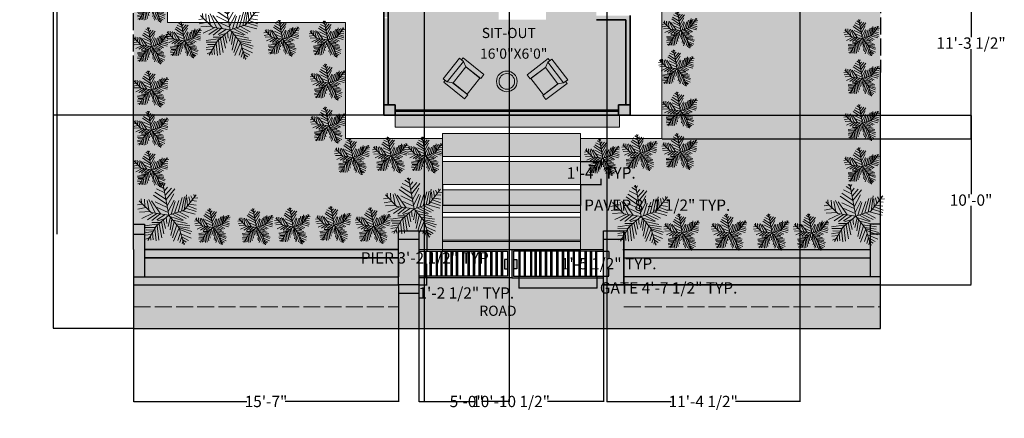
# Model space of a CAD drawing. Units: inches. Extents: x 853 to 1550, y 485 to 1596.
# Tile 1 of 18: x 853 to 1550, y 485 to 768. Entities that reach past the tile are written whole.
import ezdxf

# ---------------------------------------------------------------- set-up
doc = ezdxf.new("R2010")
doc.units = ezdxf.units.IN
doc.header["$MEASUREMENT"] = 0
doc.linetypes.add('ACAD_ISO02W100', pattern=[15, 12, -3])
for name, color, linetype, lineweight in [('A-ANNO-DIMS', 2, 'Continuous', 18), ('A-ANNO-TEXT', 250, 'Continuous', 25), ('A-AREA-IDEN', 250, 'Continuous', 18), ('A-WALL-PATT', 250, 'Continuous', 13), ('C-PROP', 8, 'ACAD_ISO02W100', 25), ('C-ROAD', 8, 'Continuous', 25), ('C-ROAD-MRKG', 7, 'ACAD_ISO02W100', 18), ('furniture', 250, 'Continuous', 18), ('L-GATE-PATT', 250, 'Continuous', 13), ('L-PAVE', 8, 'Continuous', 18), ('L-PLNT-TREE', 106, 'Continuous', 13), ('L-SITE-GATE', 250, 'Continuous', 25), ('L-SITE-WALL', 8, 'Continuous', 30), ('lawn', 106, 'Continuous', 18), ('walls', 250, 'Continuous', 35)]:
    doc.layers.add(name, color=color, linetype=linetype, lineweight=lineweight)
for name, color, linetype, lineweight, true_color in [('A-FLOR-PATT', 254, 'Continuous', 13, 0xfeeab9), ('A-FURN-PATT', 254, 'Continuous', 13, 0xfeeab9), ('C-ROAD-PATT', 250, 'Continuous', 13, 0x3d3d3d), ('L-PAVE-PATT', 9, 'Continuous', 13, 0xc7c8ca), ('L-PLNT-PATT', 85, 'Continuous', 13, 0x58ba48), ('L-SITE-WALL-PATT', 252, 'Continuous', 13, 0x939598)]:
    doc.layers.add(name, color=color, linetype=linetype, lineweight=lineweight, true_color=true_color)
doc.styles.get("Standard").update_dxf_attribs({"font": 'arial.ttf'})
doc.dimstyles.get("Standard").update_dxf_attribs({"dimtxt": 8, "dimasz": 0.18, "dimexe": 0.18, "dimexo": 0.0625, "dimgap": 0.09, "dimtad": 0, "dimtih": 1, "dimtoh": 1, "dimzin": 0, "dimdsep": 46, "dimlunit": 3, "dimtxsty": 'Standard', "dimcen": 0.09, "dimadec": 0, "dimazin": 0, "dimtfac": 1, "dimtofl": 0, "dimtmove": 0, "dimatfit": 3, "dimfxl": 1, "dimtolj": 1, "dimtzin": 0, "dimarcsym": 0})

# ---------------------------------------------------------------- blocks, each defined once
blk = doc.blocks.new('FABRIC SOFA 1S')
at = {"layer": 'furniture'}
for p, q in [((0, -15.1), (0, 15.1)), ((6, 15.1), (0, 15.1)), ((3, 18.1), (34, 18.1)), ((3, 15.1), (3, 18.1)), ((6, -15.1), (6, 15.1)), ((12, 11.8), (6, 15.1)), ((11.3, 12.1), (34, 12.1)), ((34, 12.1), (34, 18.1)), ((6, -15.1), (0, -15.1)), ((3, -18.1), (3, -15.1)), ((3, -18.1), (34, -18.1)), ((6, -15.1), (12, -11.8)), ((11.3, -12.1), (34, -12.1)), ((34, -12.1), (34, -18.1))]:
    blk.add_line(p, q, dxfattribs=at)
blk.add_lwpolyline([(12, -11.8), (12, 11.8), (33, 11.8), (33, -11.8)], close=True, dxfattribs=at)
blk = doc.blocks.new('*U18')
for p, q in [((-8.737, 47.138), (-17.069, 52.711)), ((-10.186, 53.64), (-13.084, 55.962)), ((0, 0), (-10.5, 57)), ((-9.099, 51.782), (-6.563, 55.962)), ((-3.665, 19.273), (-27.574, 35.527)), ((-5.114, 28.097), (-24.676, 40.636)), ((-7.288, 39.707), (-21.778, 46.673)), ((-7.65, 43.423), (-2.578, 49.46)), ((-5.839, 35.992), (4.667, 48.067)), ((-5.114, 27.632), (10.463, 46.673)), ((-2.941, 16.486), (8.652, 37.85)), ((27, 9), (48, 36)), ((27.127, 9.056), (31.112, 35.992)), ((44.153, 36.456), (45.239, 32.741)), ((-47.498, 19.737), (-55.83, 18.344)), ((-31.5, 4.5), (-52.5, 25.5)), ((-48.585, 21.131), (-49.309, 29.026)), ((-43.513, 28.561), (-42.427, 15.558)), ((-38.442, 26.239), (-34.819, 7.663)), ((-35.544, 28.097), (-24.314, 3.947)), ((-14.533, 2.09), (-30.834, 25.31)), ((-24.314, 23.917), (-2.941, 13.7)), ((-1.129, 6.734), (9.014, 26.704)), ((3.942, 1.625), (11.187, 24.381)), ((10.101, 3.483), (17.708, 26.239)), ((16.259, 5.805), (23.142, 31.348)), ((22.055, 7.198), (27.489, 32.277)), ((31.836, 30.883), (32.561, 16.486)), ((35.096, 32.741), (37.27, 22.524)), ((36.183, 19.737), (48.137, 17.88)), ((38.719, 34.134), (41.979, 28.561)), ((40.53, 25.775), (48.862, 24.846)), ((43.791, 29.954), (51.036, 30.883)), ((-40.615, 13.7), (-55.105, 10.913)), ((-33.37, 6.269), (-52.207, 5.34)), ((-28.299, 3.483), (-47.86, -5.805)), ((-21.416, 3.018), (-38.079, -8.128)), ((0, 0), (-31.5, 4.5)), ((-15.982, 2.09), (-30.11, -9.521)), ((0, 0), (-22.5, -19.5)), ((-6.563, 1.161), (-21.416, -8.128)), ((-20.691, 13.7), (-1.129, 4.876)), ((0, 0), (27, 9)), ((0, 0), (18, -22.5)), ((6.478, 1.625), (26.04, -8.592)), ((11.187, 3.483), (30.749, -5.805)), ((18.07, 5.805), (35.096, -3.483)), ((24.229, 7.663), (46.688, 1.625)), ((29.662, 12.307), (48.137, 6.269)), ((33.285, 16.486), (48.862, 10.913)), ((-17.431, -15.094), (-42.789, -18.809)), ((-15.257, -12.772), (-30.11, -12.772)), ((-6.563, -5.805), (-19.967, -9.985)), ((-17.069, -15.094), (-12.721, -40.172)), ((-13.446, -11.378), (-8.737, -32.741)), ((-9.461, -8.592), (-6.201, -23.453)), ((-4.752, -3.483), (-3.665, -14.629)), ((2.493, -3.019), (-1.491, -20.202)), ((1.769, -2.555), (24.229, -9.521)), ((5.029, -6.27), (2.131, -25.775)), ((9.014, -11.378), (3.58, -35.992)), ((14.085, -16.951), (6.478, -40.172)), ((7.565, -9.056), (32.198, -14.629)), ((12.274, -15.094), (36.907, -18.809)), ((-28.299, -29.026), (-42.789, -31.348)), ((-24.314, -21.596), (-42.427, -22.06)), ((-30.834, -34.135), (-42.427, -35.528)), ((-26.849, -26.24), (-40.253, -25.775)), ((-22.5, -19.5), (-37.5, -45)), ((-29.023, -30.884), (-27.936, -43.887)), ((-25.038, -23.918), (-22.865, -45.281)), ((-20.691, -18.345), (-17.793, -44.352)), ((18.07, -22.524), (8.289, -45.745)), ((20.244, -30.419), (15.897, -44.816)), ((16.259, -19.738), (36.183, -22.989)), ((18, -22.5), (27, -52.5)), ((18.433, -22.524), (40.53, -29.026)), ((19.157, -25.311), (38.719, -33.206)), ((21.331, -32.741), (39.081, -40.636)), ((-34.457, -39.708), (-40.978, -42.494)), ((-32.646, -36.921), (-31.921, -44.352)), ((22.78, -37.85), (19.519, -48.532)), ((22.78, -38.314), (34.372, -44.816)), ((24.591, -45.745), (23.142, -50.854)), ((24.591, -43.423), (30.749, -47.603)), ((26.764, -49.925), (28.213, -50.854))]:
    blk.add_line(p, q)
blk = doc.blocks.new('*D23')
at = {"layer": 'A-ANNO-DIMS', "color": 0, "lineweight": -2, "transparency": 16777216}
for p, q in [((879.97, 1474.13), (879.75, 1474.13)), ((879.93, 1473.95), (879.93, 1049.11)), ((879.93, 615.92), (879.93, 1040.76)), ((879.97, 615.74), (879.75, 615.74))]:
    blk.add_line(p, q, dxfattribs=at)
at = {"layer": 'A-ANNO-DIMS', "color": 0, "transparency": 16777216}
for points in [[(879.9, 1473.95), (879.96, 1473.95), (879.93, 1474.13)], [(879.9, 615.92), (879.96, 615.92), (879.93, 615.74)]]:
    blk.add_solid(points, dxfattribs=at)
at = {"layer": 'Defpoints', "color": 0, "transparency": 16777216}
for p in [(880.03, 1474.13), (879.93, 615.74), (880.03, 615.74)]:
    blk.add_point(p, dxfattribs=at)
at = {"layer": 'A-ANNO-DIMS', "color": 0, "transparency": 16777216, "insert": (879.93, 1044.94), "char_height": 8, "attachment_point": 5}
blk.add_mtext("\\A1;60'", dxfattribs=at)
blk = doc.blocks.new('GATE-PICKET-PANEL')
for p, q in [((0, 17.73), (0, 0)), ((1.11, 0), (1.11, 17.73)), ((3.76, 17.73), (3.76, 0)), ((4.87, 0), (4.87, 17.73)), ((8.23, 17.73), (8.23, 0)), ((9.34, 0), (9.34, 17.73)), ((11.49, 17.73), (11.49, 0)), ((12.61, 0), (12.61, 17.73)), ((14.66, 17.73), (14.66, 0)), ((15.77, 0), (15.77, 17.73)), ((18.68, 17.73), (18.68, 0)), ((19.79, 0), (19.79, 17.73)), ((22.43, 17.73), (22.43, 0)), ((23.54, 0), (23.54, 17.73)), ((26.82, 17.73), (26.82, 0)), ((27.93, 0), (27.93, 17.73)), ((30.74, 17.73), (30.74, 0)), ((31.85, 0), (31.85, 17.73)), ((34.53, 17.73), (34.53, 0)), ((35.64, 0), (35.64, 17.73)), ((38.4, 17.73), (38.4, 0)), ((39.51, 0), (39.51, 17.73)), ((42.59, 17.73), (42.59, 0)), ((43.7, 0), (43.7, 17.73)), ((46.7, 17.73), (46.7, 0)), ((47.82, 0), (47.82, 17.73)), ((50.49, 17.73), (50.49, 0)), ((51.61, 0), (51.61, 17.73)), ((54.2, 17.73), (54.2, 0)), ((55.32, 0), (55.32, 17.73))]:
    blk.add_line(p, q)
blk = doc.blocks.new('GATE-PIER')
for p, q in [((0, 38.25), (14.43, 38.25)), ((0, 0), (0, 38.25)), ((14.43, 38.25), (14.43, 0)), ((0, 32.5), (14.43, 32.5)), ((14.43, 0), (0, 0))]:
    blk.add_line(p, q)
blk = doc.blocks.new('ENTRY-PAVER')
for p, q in [((0, 16.22), (97.66, 16.22)), ((0, 0), (0, 16.22)), ((0, 16.22), (97.66, 16.22)), ((0, 0), (0, 16.22)), ((97.66, 16.22), (97.66, 0)), ((97.66, 16.22), (97.66, 0)), ((97.66, 0), (0, 0)), ((97.66, 0), (0, 0))]:
    blk.add_line(p, q)
blk = doc.blocks.new('*D47')
at = {"layer": 'A-ANNO-DIMS', "color": 0, "lineweight": -2, "transparency": 16777216}
for p, q in [((1152.25, 650.83), (1152.25, 636.06)), ((1249.91, 650.83), (1249.91, 636.06)), ((1152.43, 636.24), (1249.73, 636.24)), ((1249.91, 636.24), (1250.09, 636.24))]:
    blk.add_line(p, q, dxfattribs=at)
at = {"layer": 'A-ANNO-DIMS', "color": 0, "transparency": 16777216}
for points in [[(1152.43, 636.27), (1152.43, 636.21), (1152.25, 636.24)], [(1249.73, 636.27), (1249.73, 636.21), (1249.91, 636.24)]]:
    blk.add_solid(points, dxfattribs=at)
at = {"layer": 'Defpoints', "color": 0, "transparency": 16777216}
for p in [(1152.25, 650.89), (1249.91, 650.89), (1249.91, 636.24)]:
    blk.add_point(p, dxfattribs=at)
at = {"layer": 'A-ANNO-DIMS', "color": 0, "transparency": 16777216, "insert": (1304.18, 636.24), "char_height": 8, "attachment_point": 5}
blk.add_mtext('\\A1;PAVER 8\'-1 1/2" TYP.', dxfattribs=at)
blk = doc.blocks.new('*D48')
at = {"layer": 'A-ANNO-DIMS', "color": 0, "lineweight": -2, "transparency": 16777216}
for p, q in [((1249.97, 667.11), (1264.74, 667.11)), ((1264.56, 666.93), (1264.56, 663.11)), ((1264.56, 651.07), (1264.56, 654.89)), ((1249.97, 650.89), (1264.74, 650.89))]:
    blk.add_line(p, q, dxfattribs=at)
at = {"layer": 'A-ANNO-DIMS', "color": 0, "transparency": 16777216}
for points in [[(1264.53, 666.93), (1264.59, 666.93), (1264.56, 667.11)], [(1264.53, 651.07), (1264.59, 651.07), (1264.56, 650.89)]]:
    blk.add_solid(points, dxfattribs=at)
at = {"layer": 'Defpoints', "color": 0, "transparency": 16777216}
for p in [(1249.91, 667.11), (1264.56, 667.11), (1249.91, 650.89)]:
    blk.add_point(p, dxfattribs=at)
at = {"layer": 'A-ANNO-DIMS', "color": 0, "transparency": 16777216, "insert": (1264.56, 659), "char_height": 8, "attachment_point": 5}
blk.add_mtext('\\A1;1\'-4" TYP.', dxfattribs=at)
blk = doc.blocks.new('*D59')
at = {"layer": 'A-ANNO-DIMS', "color": 0, "lineweight": -2, "transparency": 16777216}
for p, q in [((1206.23, 585.9), (1206.23, 577.48)), ((1261.55, 585.9), (1261.55, 577.48)), ((1206.41, 577.66), (1261.37, 577.66)), ((1261.55, 577.66), (1261.73, 577.66))]:
    blk.add_line(p, q, dxfattribs=at)
at = {"layer": 'A-ANNO-DIMS', "color": 0, "transparency": 16777216}
for points in [[(1206.41, 577.69), (1206.41, 577.63), (1206.23, 577.66)], [(1261.37, 577.69), (1261.37, 577.63), (1261.55, 577.66)]]:
    blk.add_solid(points, dxfattribs=at)
at = {"layer": 'Defpoints', "color": 0, "transparency": 16777216}
for p in [(1206.23, 585.96), (1261.55, 585.96), (1261.55, 577.66)]:
    blk.add_point(p, dxfattribs=at)
at = {"layer": 'A-ANNO-DIMS', "color": 0, "transparency": 16777216, "insert": (1312.22, 577.66), "char_height": 8, "attachment_point": 5}
blk.add_mtext('\\A1;GATE 4\'-7 1/2" TYP.', dxfattribs=at)
blk = doc.blocks.new('*D60')
at = {"layer": 'A-ANNO-DIMS', "color": 0, "lineweight": -2, "transparency": 16777216}
for p, q in [((1261.61, 603.69), (1270.02, 603.69)), ((1269.84, 603.51), (1269.84, 599.05)), ((1261.61, 585.96), (1270.02, 585.96)), ((1269.84, 586.14), (1269.84, 590.6))]:
    blk.add_line(p, q, dxfattribs=at)
at = {"layer": 'A-ANNO-DIMS', "color": 0, "transparency": 16777216}
for points in [[(1269.81, 603.51), (1269.87, 603.51), (1269.84, 603.69)], [(1269.81, 586.14), (1269.87, 586.14), (1269.84, 585.96)]]:
    blk.add_solid(points, dxfattribs=at)
at = {"layer": 'Defpoints', "color": 0, "transparency": 16777216}
for p in [(1261.55, 603.69), (1269.84, 603.69), (1261.55, 585.96)]:
    blk.add_point(p, dxfattribs=at)
at = {"layer": 'A-ANNO-DIMS', "color": 0, "transparency": 16777216, "insert": (1269.84, 594.82), "char_height": 8, "attachment_point": 5}
blk.add_mtext('\\A1;1\'-5 1/2" TYP.', dxfattribs=at)
blk = doc.blocks.new('*D61')
at = {"layer": 'A-ANNO-DIMS', "color": 0, "lineweight": -2, "transparency": 16777216}
for p, q in [((1135.63, 618.05), (1141.48, 618.05)), ((1141.3, 617.87), (1141.3, 603.15)), ((1141.3, 579.98), (1141.3, 594.7)), ((1135.63, 579.8), (1141.48, 579.8))]:
    blk.add_line(p, q, dxfattribs=at)
at = {"layer": 'A-ANNO-DIMS', "color": 0, "transparency": 16777216}
for points in [[(1141.27, 617.87), (1141.33, 617.87), (1141.3, 618.05)], [(1141.27, 579.98), (1141.33, 579.98), (1141.3, 579.8)]]:
    blk.add_solid(points, dxfattribs=at)
at = {"layer": 'Defpoints', "color": 0, "transparency": 16777216}
for p in [(1135.56, 618.05), (1141.3, 618.05), (1135.56, 579.8)]:
    blk.add_point(p, dxfattribs=at)
at = {"layer": 'A-ANNO-DIMS', "color": 0, "transparency": 16777216, "insert": (1141.3, 598.92), "char_height": 8, "attachment_point": 5}
blk.add_mtext('\\A1;PIER 3\'-2 1/2" TYP.', dxfattribs=at)
blk = doc.blocks.new('*D62')
at = {"layer": 'A-ANNO-DIMS', "color": 0, "lineweight": -2, "transparency": 16777216}
for p, q in [((1121.13, 579.73), (1121.13, 573.88)), ((1135.56, 579.73), (1135.56, 573.88)), ((1121.31, 574.06), (1135.38, 574.06)), ((1135.56, 574.06), (1135.74, 574.06))]:
    blk.add_line(p, q, dxfattribs=at)
at = {"layer": 'A-ANNO-DIMS', "color": 0, "transparency": 16777216}
for points in [[(1121.31, 574.09), (1121.31, 574.03), (1121.13, 574.06)], [(1135.38, 574.09), (1135.38, 574.03), (1135.56, 574.06)]]:
    blk.add_solid(points, dxfattribs=at)
at = {"layer": 'Defpoints', "color": 0, "transparency": 16777216}
for p in [(1121.13, 579.8), (1135.56, 579.8), (1135.56, 574.06)]:
    blk.add_point(p, dxfattribs=at)
at = {"layer": 'A-ANNO-DIMS', "color": 0, "transparency": 16777216, "insert": (1169.16, 574.06), "char_height": 8, "attachment_point": 5}
blk.add_mtext('\\A1;1\'-2 1/2" TYP.', dxfattribs=at)
blk = doc.blocks.new('*D70')
at = {"layer": 'A-ANNO-DIMS', "color": 0, "lineweight": -2, "transparency": 16777216}
for p, q in [((981.87, 1426.13), (877.09, 1426.13)), ((877.27, 1425.95), (877.27, 1067.22)), ((877.27, 700.05), (877.27, 1058.77)), ((1110.88, 699.87), (877.09, 699.87))]:
    blk.add_line(p, q, dxfattribs=at)
at = {"layer": 'A-ANNO-DIMS', "color": 0, "transparency": 16777216}
for points in [[(877.24, 1425.95), (877.3, 1425.95), (877.27, 1426.13)], [(877.24, 700.05), (877.3, 700.05), (877.27, 699.87)]]:
    blk.add_solid(points, dxfattribs=at)
at = {"layer": 'Defpoints', "color": 0, "transparency": 16777216}
for p in [(981.94, 1426.13), (877.27, 699.87), (1110.94, 699.87)]:
    blk.add_point(p, dxfattribs=at)
at = {"layer": 'A-ANNO-DIMS', "color": 0, "transparency": 16777216, "insert": (877.27, 1063), "char_height": 8, "attachment_point": 5}
blk.add_mtext('\\A1;60\'-6 1/2"', dxfattribs=at)
blk = doc.blocks.new('*D71')
at = {"layer": 'A-ANNO-DIMS', "color": 0, "lineweight": -2, "transparency": 16777216}
for p, q in [((933.87, 1474.13), (877.09, 1474.13)), ((877.27, 1473.95), (877.27, 1015.66)), ((877.27, 549.16), (877.27, 1007.45)), ((933.87, 548.98), (877.09, 548.98))]:
    blk.add_line(p, q, dxfattribs=at)
at = {"layer": 'A-ANNO-DIMS', "color": 0, "transparency": 16777216}
for points in [[(877.24, 1473.95), (877.3, 1473.95), (877.27, 1474.13)], [(877.24, 549.16), (877.3, 549.16), (877.27, 548.98)]]:
    blk.add_solid(points, dxfattribs=at)
at = {"layer": 'Defpoints', "color": 0, "transparency": 16777216}
for p in [(877.27, 1474.13), (933.94, 1474.13), (933.94, 548.98)]:
    blk.add_point(p, dxfattribs=at)
at = {"layer": 'A-ANNO-DIMS', "color": 0, "transparency": 16777216, "insert": (877.27, 1011.55), "char_height": 8, "attachment_point": 5}
blk.add_mtext('\\A1;77\'-1"', dxfattribs=at)
blk = doc.blocks.new('*D72')
at = {"layer": 'A-ANNO-DIMS', "color": 0, "lineweight": -2, "transparency": 16777216}
for p, q in [((1139.44, 1321.07), (1139.44, 497.1)), ((1199.44, 1321.07), (1199.44, 497.1)), ((1139.62, 497.28), (1158.71, 497.28)), ((1199.26, 497.28), (1180.16, 497.28))]:
    blk.add_line(p, q, dxfattribs=at)
at = {"layer": 'A-ANNO-DIMS', "color": 0, "transparency": 16777216}
for points in [[(1139.62, 497.31), (1139.62, 497.25), (1139.44, 497.28)], [(1199.26, 497.31), (1199.26, 497.25), (1199.44, 497.28)]]:
    blk.add_solid(points, dxfattribs=at)
at = {"layer": 'Defpoints', "color": 0, "transparency": 16777216}
for p in [(1139.44, 1321.13), (1199.44, 1321.13), (1199.44, 497.28)]:
    blk.add_point(p, dxfattribs=at)
at = {"layer": 'A-ANNO-DIMS', "color": 0, "transparency": 16777216, "insert": (1169.44, 497.28), "char_height": 8, "attachment_point": 5}
blk.add_mtext('\\A1;5\'-0"', dxfattribs=at)
blk = doc.blocks.new('*D74')
at = {"layer": 'A-ANNO-DIMS', "color": 0, "lineweight": -2, "transparency": 16777216}
for p, q in [((1268.44, 863.57), (1268.44, 497.1)), ((1404.94, 863.57), (1404.94, 497.1)), ((1268.62, 497.28), (1313.91, 497.28)), ((1404.76, 497.28), (1359.46, 497.28))]:
    blk.add_line(p, q, dxfattribs=at)
at = {"layer": 'A-ANNO-DIMS', "color": 0, "transparency": 16777216}
for points in [[(1268.62, 497.31), (1268.62, 497.25), (1268.44, 497.28)], [(1404.76, 497.31), (1404.76, 497.25), (1404.94, 497.28)]]:
    blk.add_solid(points, dxfattribs=at)
at = {"layer": 'Defpoints', "color": 0, "transparency": 16777216}
for p in [(1268.44, 863.63), (1404.94, 863.63), (1404.94, 497.28)]:
    blk.add_point(p, dxfattribs=at)
at = {"layer": 'A-ANNO-DIMS', "color": 0, "transparency": 16777216, "insert": (1336.69, 497.28), "char_height": 8, "attachment_point": 5}
blk.add_mtext('\\A1;11\'-4 1/2"', dxfattribs=at)
blk = doc.blocks.new('*D76')
at = {"layer": 'A-ANNO-DIMS', "color": 0, "lineweight": -2, "transparency": 16777216}
for p, q in [((1135.56, 579.73), (1135.56, 497.1)), ((1266.06, 579.73), (1266.06, 497.1)), ((1135.74, 497.28), (1174.93, 497.28)), ((1265.88, 497.28), (1226.69, 497.28))]:
    blk.add_line(p, q, dxfattribs=at)
at = {"layer": 'A-ANNO-DIMS', "color": 0, "transparency": 16777216}
for points in [[(1135.74, 497.31), (1135.74, 497.25), (1135.56, 497.28)], [(1265.88, 497.31), (1265.88, 497.25), (1266.06, 497.28)]]:
    blk.add_solid(points, dxfattribs=at)
at = {"layer": 'Defpoints', "color": 0, "transparency": 16777216}
for p in [(1135.56, 579.8), (1266.06, 579.8), (1266.06, 497.28)]:
    blk.add_point(p, dxfattribs=at)
at = {"layer": 'A-ANNO-DIMS', "color": 0, "transparency": 16777216, "insert": (1200.81, 497.28), "char_height": 8, "attachment_point": 5}
blk.add_mtext('\\A1;10\'-10 1/2"', dxfattribs=at)
blk = doc.blocks.new('*D77')
at = {"layer": 'A-ANNO-DIMS', "color": 0, "lineweight": -2, "transparency": 16777216}
for p, q in [((933.94, 579.73), (933.94, 497.1)), ((1121.13, 579.73), (1121.13, 497.1)), ((934.12, 497.28), (1014.08, 497.28)), ((1120.95, 497.28), (1040.99, 497.28))]:
    blk.add_line(p, q, dxfattribs=at)
at = {"layer": 'A-ANNO-DIMS', "color": 0, "transparency": 16777216}
for points in [[(934.12, 497.31), (934.12, 497.25), (933.94, 497.28)], [(1120.95, 497.31), (1120.95, 497.25), (1121.13, 497.28)]]:
    blk.add_solid(points, dxfattribs=at)
at = {"layer": 'Defpoints', "color": 0, "transparency": 16777216}
for p in [(933.94, 579.8), (1121.13, 579.8), (1121.13, 497.28)]:
    blk.add_point(p, dxfattribs=at)
at = {"layer": 'A-ANNO-DIMS', "color": 0, "transparency": 16777216, "insert": (1027.53, 497.28), "char_height": 8, "attachment_point": 5}
blk.add_mtext('\\A1;15\'-7"', dxfattribs=at)
blk = doc.blocks.new('*D78')
at = {"layer": 'A-ANNO-DIMS', "color": 0, "lineweight": -2, "transparency": 16777216}
for p, q in [((1284.98, 699.87), (1526.24, 699.87)), ((1526.06, 699.69), (1526.06, 644.01)), ((1526.06, 579.98), (1526.06, 635.66)), ((1266.12, 579.8), (1526.24, 579.8))]:
    blk.add_line(p, q, dxfattribs=at)
at = {"layer": 'A-ANNO-DIMS', "color": 0, "transparency": 16777216}
for points in [[(1526.03, 699.69), (1526.09, 699.69), (1526.06, 699.87)], [(1526.03, 579.98), (1526.09, 579.98), (1526.06, 579.8)]]:
    blk.add_solid(points, dxfattribs=at)
at = {"layer": 'Defpoints', "color": 0, "transparency": 16777216}
for p in [(1284.92, 699.87), (1526.06, 699.87), (1266.06, 579.8)]:
    blk.add_point(p, dxfattribs=at)
at = {"layer": 'A-ANNO-DIMS', "color": 0, "transparency": 16777216, "insert": (1526.06, 639.83), "char_height": 8, "attachment_point": 5}
blk.add_mtext('\\A1;10\'-0"', dxfattribs=at)
blk = doc.blocks.new('*D80')
at = {"layer": 'A-ANNO-DIMS', "color": 0, "lineweight": -2, "transparency": 16777216}
for p, q in [((1307.55, 818.63), (1526.24, 818.63)), ((1526.06, 818.45), (1526.06, 755.21)), ((1526.06, 683.5), (1526.06, 746.75)), ((1307.55, 683.32), (1526.24, 683.32))]:
    blk.add_line(p, q, dxfattribs=at)
at = {"layer": 'A-ANNO-DIMS', "color": 0, "transparency": 16777216}
for points in [[(1526.03, 818.45), (1526.09, 818.45), (1526.06, 818.63)], [(1526.03, 683.5), (1526.09, 683.5), (1526.06, 683.32)]]:
    blk.add_solid(points, dxfattribs=at)
at = {"layer": 'Defpoints', "color": 0, "transparency": 16777216}
for p in [(1307.49, 818.63), (1526.06, 818.63), (1307.49, 683.32)]:
    blk.add_point(p, dxfattribs=at)
at = {"layer": 'A-ANNO-DIMS', "color": 0, "transparency": 16777216, "insert": (1526.06, 750.98), "char_height": 8, "attachment_point": 5}
blk.add_mtext('\\A1;11\'-3 1/2"', dxfattribs=at)

msp = doc.modelspace()

# ---------------------------------------------------------------- hatches: boundary and pattern name
at = {"layer": 'A-FLOR-PATT'}
h = msp.add_hatch(color=256, dxfattribs=at)
h.dxf.hatch_style = 1
h.paths.add_polyline_path([(1113.94, 788.629), (1110.94, 788.629), (1110.94, 769.463), (1113.94, 769.463)])
h.paths.add_polyline_path([(1113.94, 768.501), (1110.94, 768.501), (1110.94, 707.356), (1113.94, 707.356)])
h.paths.add_polyline_path([(1276.896, 702.868), (1118.963, 702.868), (1118.963, 699.868), (1276.896, 699.868)])
h.paths.add_polyline_path([(1284.919, 770.496), (1261.179, 770.496), (1261.179, 767.496), (1281.919, 767.496), (1281.919, 707.356), (1284.919, 707.356)])
h = msp.add_hatch(color=256, dxfattribs=at)
h.dxf.hatch_style = 1
h.paths.add_polyline_path([(1281.919, 767.496), (1261.179, 767.496), (1113.94, 767.629), (1113.94, 707.356), (1118.963, 707.356), (1118.963, 702.868), (1276.896, 702.868), (1276.896, 707.356), (1281.919, 707.356)])
at = {"layer": 'A-FURN-PATT'}
h = msp.add_hatch(color=256, dxfattribs=at)
h.dxf.hatch_style = 1
h.paths.add_polyline_path([(1168.748, 734.08), (1159.864, 722.847), (1169.901, 714.908), (1178.786, 726.14)])
h.paths.add_polyline_path([(1168.748, 734.08), (1167.156, 737.961), (1155.72, 723.502), (1159.864, 722.847)])
h.paths.add_polyline_path([(1167.156, 737.961), (1164.289, 740.23), (1152.852, 725.771), (1155.72, 723.502)])
h.paths.add_polyline_path([(1159.403, 722.92), (1155.72, 723.502), (1154.286, 724.637), (1153.152, 723.203), (1167.969, 711.483), (1170.238, 714.35)])
h.paths.add_polyline_path([(1166.857, 740.529), (1165.723, 739.095), (1167.156, 737.961), (1168.572, 734.511), (1179.406, 725.941), (1181.674, 728.809)])
h = msp.add_hatch(color=256, dxfattribs=at)
h.dxf.hatch_style = 1
h.paths.add_polyline_path([(1225.103, 733.585), (1214.928, 725.823), (1223.614, 714.436), (1233.789, 722.198)])
h.paths.add_polyline_path([(1225.288, 734.013), (1226.763, 737.438), (1228.217, 738.547), (1227.108, 740), (1212.087, 728.542), (1214.305, 725.635)])
h.paths.add_polyline_path([(1240.506, 722.436), (1239.398, 723.889), (1237.944, 722.78), (1234.251, 722.263), (1223.268, 713.885), (1225.486, 710.978)])
h.paths.add_polyline_path([(1226.763, 737.438), (1225.103, 733.585), (1233.789, 722.198), (1237.944, 722.78)])
h.paths.add_polyline_path([(1229.67, 739.656), (1226.763, 737.438), (1237.944, 722.78), (1240.851, 724.998)])
h = msp.add_hatch(color=256, dxfattribs=at)
h.dxf.hatch_style = 1
h.paths.add_polyline_path([(1192.315, 723.874, 1), (1203.335, 723.874, 1)], flags=0)
h.paths.add_polyline_path([(1190.506, 723.874, 1), (1205.144, 723.874, 1)])
h.paths.add_polyline_path([(1203.335, 723.874, -1), (1192.315, 723.874, -1)], flags=16)
h = msp.add_hatch(color=256, dxfattribs=at)
h.dxf.hatch_style = 1
h.paths.add_polyline_path([(1192.315, 723.874, 1), (1203.335, 723.874, 1)])
at = {"layer": 'A-WALL-PATT'}
h = msp.add_hatch(color=256, dxfattribs=at)
h.dxf.hatch_style = 1
h.paths.add_polyline_path([(990.937, 1111.29), (981.937, 1111.29), (981.937, 1044.136), (984.946, 1044.136), (990.937, 1044.136), (990.937, 1072.129), (1045.609, 1072.129, -0.0272078), (1045.453, 1074.983), (1045.453, 1076.629), (990.937, 1076.629)], flags=17)
h.paths.add_polyline_path([(1091.437, 1072.129), (1139.437, 1072.129), (1139.437, 1206.521), (1134.937, 1206.521), (1134.937, 1076.629), (1071.734, 1076.629), (1071.734, 1074.983), (1071.734, 1072.129), (1086.937, 1072.129), (1086.937, 1012.129), (990.937, 1012.129), (981.937, 1012.129), (981.937, 944.409), (990.937, 944.409), (990.937, 1007.629), (1091.437, 1007.629)])
h.paths.add_polyline_path([(990.937, 872.981), (981.937, 872.981), (981.937, 788.629), (990.937, 788.629)])
h.paths.add_polyline_path([(1014.605, 800.886), (990.937, 800.886), (990.937, 796.386), (1014.605, 796.386)])
h.paths.add_polyline_path([(1134.937, 793.129), (1090.727, 793.129), (1090.727, 788.629), (1134.937, 788.629)])
h.paths.add_polyline_path([(1139.437, 800.892), (1134.937, 800.892), (1134.937, 788.629), (1113.94, 788.629), (1113.94, 767.629), (1139.437, 767.629), (1191.938, 767.629), (1191.938, 772.657), (1191.938, 776.629), (1139.437, 776.629)])
h.paths.add_polyline_path([(1131.331, 781.621), (1131.331, 775.236), (1118.809, 775.236), (1118.809, 781.621)], flags=16)
h.paths.add_polyline_path([(1131.331, 781.621), (1118.809, 781.621), (1118.809, 775.236), (1131.331, 775.236)], flags=0)
h.paths.add_polyline_path([(1118.963, 707.356), (1110.94, 707.356), (1110.94, 699.868), (1118.963, 699.868)])
h.paths.add_polyline_path([(1284.919, 707.356), (1276.896, 707.356), (1276.896, 699.868), (1284.919, 699.868)])
h.paths.add_polyline_path([(1293.812, 863.629), (1268.437, 863.629), (1268.437, 984.936), (1308.937, 984.936), (1308.937, 996.627), (1304.437, 996.627), (1304.437, 989.436), (1263.937, 989.436), (1263.937, 863.629), (1215.364, 863.629), (1215.364, 854.629), (1252.179, 854.629), (1252.179, 776.629), (1225.216, 776.629, -0.0297134), (1225.453, 772.657), (1225.453, 767.629), (1261.179, 767.629), (1261.179, 854.629), (1293.812, 854.629)])
h.paths.add_polyline_path([(1176.151, 863.629), (1139.437, 863.629), (1139.437, 854.629), (1176.151, 854.629)])
h.paths.add_polyline_path([(1134.937, 863.629), (1109.834, 863.629), (1109.834, 859.129), (1134.937, 859.129)])
h.paths.add_polyline_path([(1148.879, 950.672), (1144.374, 950.672), (1144.374, 874.094), (1148.879, 874.094)])
h.paths.add_polyline_path([(1079.778, 863.629), (990.937, 863.629), (990.937, 859.129), (1079.778, 859.129)])
at = {"layer": 'C-ROAD-PATT'}
h = msp.add_hatch(color=256, dxfattribs=at)
h.dxf.hatch_style = 1
h.paths.add_polyline_path([(1461.937, 579.797), (1280.493, 579.797), (1266.059, 579.797), (1266.059, 584.715), (1201.399, 584.715), (1135.564, 584.715), (1135.564, 579.797), (1121.13, 579.797), (933.937, 579.797), (933.937, 548.979), (1461.937, 548.979)])
at = {"layer": 'L-GATE-PATT'}
h = msp.add_hatch(color=256, dxfattribs=at)
h.dxf.hatch_style = 1
h.paths.add_polyline_path([(1152.247, 604.895), (1135.564, 604.895), (1135.564, 603.686), (1152.247, 603.686)], flags=0)
h.paths.add_polyline_path([(1199.458, 604.895), (1152.247, 604.895), (1152.247, 603.686), (1198.395, 603.686), (1198.395, 585.96), (1135.564, 585.96), (1135.564, 584.715), (1199.458, 584.715)])
h = msp.add_hatch(color=256, dxfattribs=at)
h.dxf.hatch_style = 1
h.paths.add_polyline_path([(1152.247, 604.895), (1135.564, 604.895), (1135.564, 603.686), (1152.247, 603.686)])
h.paths.add_polyline_path([(1249.908, 604.895), (1201.399, 604.895), (1201.399, 584.715), (1266.059, 584.715), (1266.059, 585.96), (1202.558, 585.96), (1202.558, 603.686), (1249.908, 603.686)])
h.paths.add_polyline_path([(1266.059, 604.895), (1249.908, 604.895), (1249.908, 603.686), (1266.059, 603.686)], flags=17)
h = msp.add_hatch(color=256, dxfattribs=at)
h.dxf.hatch_style = 1
h.paths.add_polyline_path([(1140.689, 603.686), (1139.578, 603.686), (1139.578, 585.96), (1140.689, 585.96)])
h.paths.add_polyline_path([(1144.445, 603.686), (1143.333, 603.686), (1143.333, 585.96), (1144.445, 585.96)])
h.paths.add_polyline_path([(1148.917, 603.686), (1147.805, 603.686), (1147.805, 585.96), (1148.917, 585.96)])
h.paths.add_polyline_path([(1152.183, 603.686), (1151.071, 603.686), (1151.071, 585.96), (1152.183, 585.96)])
h.paths.add_polyline_path([(1155.349, 603.686), (1154.237, 603.686), (1154.237, 585.96), (1155.349, 585.96)])
h.paths.add_polyline_path([(1159.369, 603.686), (1158.257, 603.686), (1158.257, 585.96), (1159.369, 585.96)])
h.paths.add_polyline_path([(1163.123, 603.686), (1162.011, 603.686), (1162.011, 585.96), (1163.123, 585.96)])
h.paths.add_polyline_path([(1167.511, 603.686), (1166.399, 603.686), (1166.399, 585.96), (1167.511, 585.96)])
h.paths.add_polyline_path([(1171.428, 603.686), (1170.317, 603.686), (1170.317, 585.96), (1171.428, 585.96)])
h.paths.add_polyline_path([(1175.218, 603.686), (1174.107, 603.686), (1174.107, 585.96), (1175.218, 585.96)])
h.paths.add_polyline_path([(1179.089, 603.686), (1177.977, 603.686), (1177.977, 585.96), (1179.089, 585.96)])
h.paths.add_polyline_path([(1183.282, 603.686), (1182.17, 603.686), (1182.17, 585.96), (1183.282, 585.96)])
h.paths.add_polyline_path([(1187.394, 603.686), (1186.283, 603.686), (1186.283, 585.96), (1187.394, 585.96)])
h.paths.add_polyline_path([(1191.184, 603.686), (1190.073, 603.686), (1190.073, 585.96), (1191.184, 585.96)])
h.paths.add_polyline_path([(1194.894, 603.686), (1193.782, 603.686), (1193.782, 585.96), (1194.894, 585.96)])
h.paths.add_polyline_path([(1198.395, 597.743), (1196.19, 597.743), (1196.19, 591.079), (1198.395, 591.079)])
h.paths.add_polyline_path([(1204.784, 597.743), (1202.558, 597.743), (1202.558, 591.079), (1204.784, 591.079)])
h.paths.add_polyline_path([(1207.342, 603.686), (1206.23, 603.686), (1206.23, 585.96), (1207.342, 585.96)])
h.paths.add_polyline_path([(1211.097, 603.686), (1209.985, 603.686), (1209.985, 585.96), (1211.097, 585.96)])
h.paths.add_polyline_path([(1215.569, 603.686), (1214.458, 603.686), (1214.458, 585.96), (1215.569, 585.96)])
h.paths.add_polyline_path([(1218.835, 603.686), (1217.724, 603.686), (1217.724, 585.96), (1218.835, 585.96)])
h.paths.add_polyline_path([(1222.001, 603.686), (1220.89, 603.686), (1220.89, 585.96), (1222.001, 585.96)])
h.paths.add_polyline_path([(1226.021, 603.686), (1224.91, 603.686), (1224.91, 585.96), (1226.021, 585.96)])
h.paths.add_polyline_path([(1229.775, 603.686), (1228.664, 603.686), (1228.664, 585.96), (1229.775, 585.96)])
h.paths.add_polyline_path([(1234.163, 603.686), (1233.052, 603.686), (1233.052, 585.96), (1234.163, 585.96)])
h.paths.add_polyline_path([(1238.081, 603.686), (1236.969, 603.686), (1236.969, 585.96), (1238.081, 585.96)])
h.paths.add_polyline_path([(1241.871, 603.686), (1240.759, 603.686), (1240.759, 585.96), (1241.871, 585.96)])
h.paths.add_polyline_path([(1245.741, 603.686), (1244.63, 603.686), (1244.63, 585.96), (1245.741, 585.96)])
h.paths.add_polyline_path([(1249.934, 603.686), (1248.823, 603.686), (1248.823, 585.96), (1249.934, 585.96)])
h.paths.add_polyline_path([(1254.047, 603.686), (1252.935, 603.686), (1252.935, 585.96), (1254.047, 585.96)])
h.paths.add_polyline_path([(1257.837, 603.686), (1256.725, 603.686), (1256.725, 585.96), (1257.837, 585.96)])
h.paths.add_polyline_path([(1261.546, 603.686), (1260.434, 603.686), (1260.434, 585.96), (1261.546, 585.96)])
at = {"layer": 'L-PAVE-PATT'}
h = msp.add_hatch(color=256, dxfattribs=at)
h.dxf.hatch_style = 1
h.paths.add_polyline_path([(1277.428, 699.868), (1118.963, 699.868), (1118.963, 691.576), (1277.428, 691.576)])
h.paths.add_polyline_path([(1249.908, 686.983), (1152.247, 686.983), (1152.247, 670.763), (1249.908, 670.763)])
h.paths.add_polyline_path([(1249.908, 667.113), (1152.247, 667.113), (1152.247, 650.893), (1249.908, 650.893)])
h.paths.add_polyline_path([(1249.908, 647.197), (1152.247, 647.197), (1152.247, 630.977), (1249.908, 630.977)])
h.paths.add_polyline_path([(1249.908, 627.676), (1152.247, 627.676), (1152.247, 611.456), (1249.908, 611.456)])
h = msp.add_hatch(color=256, dxfattribs=at)
h.dxf.hatch_style = 1
h.paths.add_polyline_path([(1249.908, 610.626), (1152.247, 610.626), (1152.247, 604.895), (1201.399, 604.895), (1249.908, 604.895)])
at = {"layer": 'L-PLNT-PATT'}
h = msp.add_hatch(color=256, dxfattribs=at)
h.dxf.hatch_style = 1
h.paths.add_polyline_path([(1461.937, 1474.129), (933.937, 1474.129), (933.937, 730.129), (933.937, 622.891), (941.686, 622.891), (941.686, 604.895), (957.937, 604.895), (957.937, 1450.129), (1437.937, 1450.129), (1437.937, 604.895), (1454.646, 604.895), (1454.646, 622.891), (1461.937, 622.891), (1461.937, 734.988)])
h = msp.add_hatch(color=256, dxfattribs=at)
h.dxf.hatch_style = 1
h.paths.add_polyline_path([(1083.746, 765.455), (957.937, 765.455), (957.937, 604.895), (1121.13, 604.895), (1121.13, 618.052), (1135.564, 618.052), (1135.564, 604.895), (1152.247, 604.895), (1152.247, 610.626), (1152.247, 683.324), (1083.746, 683.324)])
h.paths.add_polyline_path([(1437.937, 818.629), (1307.486, 818.629), (1307.486, 683.324), (1249.908, 683.324), (1249.908, 667.104), (1249.908, 604.895), (1266.059, 604.895), (1266.059, 618.052), (1280.493, 618.052), (1280.493, 604.895), (1437.937, 604.895)])
at = {"layer": 'L-SITE-WALL-PATT'}
h = msp.add_hatch(color=256, dxfattribs=at)
h.dxf.hatch_style = 1
h.paths.add_polyline_path([(941.686, 615.743), (933.937, 615.743), (933.937, 604.895), (933.937, 585.575), (941.686, 585.575)])
h.paths.add_polyline_path([(941.686, 622.891), (933.937, 622.891), (933.937, 615.743), (941.686, 615.743)])
h.paths.add_polyline_path([(1121.13, 585.575), (933.937, 585.575), (933.937, 579.797), (1121.13, 579.797)])
h.paths.add_polyline_path([(1121.13, 604.895), (941.686, 604.895), (941.686, 598.924), (1121.13, 598.924)])
h.paths.add_polyline_path([(1135.564, 612.293), (1121.13, 612.293), (1121.13, 579.797), (1135.564, 579.797)])
h.paths.add_polyline_path([(1135.564, 618.052), (1121.13, 618.052), (1121.13, 612.293), (1135.564, 612.293)])
h.paths.add_polyline_path([(1280.493, 612.293), (1266.059, 612.293), (1266.059, 579.797), (1280.493, 579.797)])
h.paths.add_polyline_path([(1280.493, 618.052), (1266.059, 618.052), (1266.059, 612.293), (1278.06, 612.293), (1279.514, 612.914), (1280.493, 614.579)])
h.paths.add_polyline_path([(1461.937, 585.575), (1280.493, 585.575), (1280.493, 579.797), (1461.937, 579.797)])
h.paths.add_polyline_path([(1454.646, 604.895), (1280.493, 604.895), (1280.493, 598.924), (1454.646, 598.924)])
h.paths.add_polyline_path([(1461.937, 615.743), (1454.646, 615.743), (1454.646, 585.575), (1461.937, 585.575)])
h.paths.add_polyline_path([(1454.646, 617.309), (1454.646, 615.743), (1458.525, 615.743)], flags=17)
h.paths.add_polyline_path([(1461.937, 622.891), (1454.646, 622.891), (1454.646, 617.309), (1458.525, 615.743), (1461.937, 615.743)])
h = msp.add_hatch(color=256, dxfattribs=at)
h.dxf.hatch_style = 1
h.paths.add_polyline_path([(1280.493, 614.579), (1280.493, 618.052), (1266.059, 618.052), (1266.059, 612.293), (1279.148, 612.293)])
h.paths.add_polyline_path([(1280.493, 614.579), (1279.148, 612.293), (1280.493, 612.293)], flags=17)
h = msp.add_hatch(color=256, dxfattribs=at)
h.dxf.hatch_style = 1
h.paths.add_polyline_path([(1121.13, 598.924), (941.686, 598.924), (941.686, 585.575), (1121.13, 585.575)])
h.paths.add_polyline_path([(1454.646, 598.924), (1280.493, 598.924), (1280.493, 585.575), (1454.646, 585.575)])

# ---------------------------------------------------------------- linework, layer by layer
at = {"layer": 'C-PROP'}
for p, q in [((933.937, 730.129), (933.937, 1474.129)), ((1461.937, 1474.129), (1461.937, 730.129))]:
    msp.add_line(p, q, dxfattribs=at)
at = {"layer": 'C-ROAD'}
for p, q in [((933.937, 579.797), (933.937, 548.979)), ((1461.937, 548.979), (1461.937, 579.797)), ((933.937, 548.979), (1461.937, 548.979))]:
    msp.add_line(p, q, dxfattribs=at)
at = {"layer": 'C-ROAD-MRKG'}
for p, q in [((933.937, 564.388), (1121.13, 564.388)), ((1280.493, 564.388), (1461.937, 564.388))]:
    msp.add_line(p, q, dxfattribs=at)
at = {"layer": 'furniture'}
for radius in [7.319, 7.319, 5.51]:
    msp.add_circle((1197.825, 723.874), radius, dxfattribs=at)
at = {"layer": 'L-PAVE'}
for p, q in [((1118.963, 699.868), (1118.963, 691.717)), ((1118.963, 699.727), (1118.963, 691.576)), ((1276.896, 699.868), (1284.919, 699.868)), ((1277.428, 691.576), (1277.428, 699.868)), ((1118.963, 691.576), (1277.428, 691.576)), ((1152.247, 667.104), (1152.247, 683.324)), ((1249.908, 683.324), (1249.908, 667.104)), ((1152.247, 667.104), (1249.908, 667.104)), ((1152.247, 650.885), (1152.247, 667.104)), ((1249.908, 667.104), (1249.908, 650.885)), ((1249.908, 650.885), (1152.247, 650.885)), ((1152.247, 647.197), (1249.908, 647.197)), ((1152.247, 630.977), (1152.247, 647.197)), ((1249.908, 647.197), (1249.908, 630.977)), ((1249.908, 630.977), (1152.247, 630.977)), ((1152.247, 610.626), (1249.908, 610.626)), ((1152.247, 603.686), (1152.247, 610.626)), ((1249.908, 610.626), (1249.908, 603.686))]:
    msp.add_line(p, q, dxfattribs=at)
at = {"layer": 'L-SITE-GATE'}
for p, q in [((1135.564, 603.686), (1198.395, 603.686)), ((1152.247, 604.895), (1201.399, 604.895)), ((1198.395, 603.686), (1198.395, 585.96)), ((1199.458, 604.895), (1199.458, 584.715)), ((1201.399, 604.895), (1201.399, 584.715)), ((1201.399, 604.895), (1249.908, 604.895)), ((1266.059, 603.686), (1202.558, 603.686)), ((1202.558, 603.686), (1202.558, 585.96)), ((1198.395, 597.743), (1196.19, 597.743)), ((1196.19, 597.743), (1196.19, 591.079)), ((1202.558, 597.743), (1204.784, 597.743)), ((1204.784, 597.743), (1204.784, 591.079)), ((1198.395, 585.96), (1135.564, 585.96)), ((1139.578, 585.96), (1140.689, 585.96)), ((1196.19, 591.079), (1198.395, 591.079)), ((1204.784, 591.079), (1202.558, 591.079)), ((1202.558, 585.96), (1266.059, 585.96)), ((1201.399, 584.715), (1135.564, 584.715)), ((1201.399, 584.715), (1266.059, 584.715))]:
    msp.add_line(p, q, dxfattribs=at)
at = {"layer": 'L-SITE-WALL'}
for p, q in [((1461.937, 579.797), (1461.937, 734.988)), ((933.937, 604.895), (933.937, 730.129)), ((933.937, 622.891), (941.686, 622.891)), ((941.686, 622.891), (941.686, 585.575)), ((1461.937, 622.891), (1454.646, 622.891)), ((1454.646, 622.891), (1454.646, 585.575)), ((933.937, 615.743), (941.686, 615.743)), ((1266.059, 612.293), (1266.059, 618.052)), ((1266.059, 618.052), (1280.493, 618.052)), ((1280.493, 579.797), (1280.493, 618.052)), ((1461.937, 615.743), (1454.646, 615.743)), ((933.937, 604.895), (933.937, 579.797)), ((1121.13, 604.895), (941.686, 604.895)), ((941.686, 604.895), (1121.13, 604.895)), ((1121.13, 598.924), (941.686, 598.924)), ((941.686, 598.924), (1121.13, 598.924)), ((941.686, 598.924), (941.686, 585.575)), ((1121.13, 598.924), (1121.13, 585.575)), ((1279.96, 604.895), (1454.646, 604.895)), ((1280.493, 604.895), (1454.646, 604.895)), ((1280.493, 598.924), (1454.646, 598.924)), ((933.937, 585.575), (1121.13, 585.575)), ((941.686, 585.575), (1121.13, 585.575)), ((1461.937, 585.575), (1280.493, 585.575)), ((933.937, 579.797), (1121.13, 579.797)), ((1461.937, 579.797), (1280.493, 579.797))]:
    msp.add_line(p, q, dxfattribs=at)
at = {"layer": 'lawn'}
for p, q in [((957.937, 765.455), (957.937, 1450.129)), ((1307.486, 818.629), (1307.486, 683.324)), ((957.937, 765.455), (1083.746, 765.455)), ((1083.746, 765.455), (1083.746, 683.324)), ((1083.746, 683.324), (1152.247, 683.324)), ((1152.247, 683.324), (1152.247, 604.895)), ((1307.486, 683.324), (1249.908, 683.324)), ((1249.908, 683.324), (1249.908, 604.895)), ((1152.247, 604.895), (1135.564, 604.895)), ((1249.908, 604.895), (1266.059, 604.895))]:
    msp.add_line(p, q, dxfattribs=at)
at = {"layer": 'walls'}
for p, q in [((1110.94, 788.629), (1110.94, 699.868)), ((1113.94, 788.629), (1113.94, 707.356)), ((1261.179, 767.496), (1281.919, 767.496)), ((1281.919, 767.496), (1281.919, 707.356)), ((1284.919, 770.496), (1284.919, 699.868)), ((1110.94, 707.356), (1118.963, 707.356)), ((1118.963, 707.356), (1118.963, 699.868)), ((1118.963, 703.612), (1276.896, 703.612)), ((1284.919, 707.356), (1276.896, 707.356)), ((1276.896, 707.356), (1276.896, 699.868)), ((1284.919, 699.868), (1110.94, 699.868)), ((1276.896, 702.868), (1118.963, 702.868))]:
    msp.add_line(p, q, dxfattribs=at)

# ---------------------------------------------------------------- block references
at = {"layer": 'furniture', "yscale": 0.6094251026746103, "zscale": 0.6094251026746103}
for p, xscale, rotation in [((1158.57, 733), 0.6094251026746103, 321.6570261001913), ((1235.261, 732.327), -0.6094251026746103, 37.33676882741484)]:
    msp.add_blockref('FABRIC SOFA 1S', p, dxfattribs=dict(at, xscale=xscale, rotation=rotation))
at = {"layer": 'L-PAVE'}
for p in [(1152.247, 670.763), (1152.247, 650.893), (1152.247, 630.977), (1152.247, 611.456)]:
    msp.add_blockref('ENTRY-PAVER', p, dxfattribs=at)
at = {"layer": 'L-PLNT-TREE'}
for p, xscale, yscale, zscale in [((946.691, 777.957), 0.2357951711934384, 0.2357951711934384, 0.2357951711934384), ((1002.291, 760.365), 0.3996992985476591, 0.3996992985476591, 0.3996992985476591), ((1320.889, 759.87), 0.2357951711934384, 0.2357951711934384, 0.2357951711934384), ((969.924, 752.634), 0.2357951711934384, 0.2357951711934384, 0.2357951711934384), ((1039.277, 753.845), 0.2357951711934384, 0.2357951711934384, 0.2357951711934384), ((1071.152, 753.204), 0.2357951711934384, 0.2357951711934384, 0.2357951711934384), ((1449.245, 754.254), 0.2357951711934384, 0.2357951711934384, 0.2357951711934384), ((946.691, 748.526), 0.2357951711934384, 0.2357951711934384, 0.2357951711934384), ((1318.241, 732.819), 0.2357951711934384, 0.2357951711934384, 0.2357951711934384), ((1449.245, 725.826), 0.2357951711934384, 0.2357951711934384, 0.2357951711934384), ((946.691, 717.934), 0.2357951711934384, 0.2357951711934384, 0.2357951711934384), ((1071.896, 722.755), 0.2357951711934384, 0.2357951711934384, 0.2357951711934384), ((1320.547, 703.02), 0.2357951711934384, 0.2357951711934384, 0.2357951711934384), ((1071.921, 692.37), 0.2357951711934384, 0.2357951711934384, 0.2357951711934384), ((1449.245, 694.183), 0.2357951711934384, 0.2357951711934384, 0.2357951711934384), ((946.691, 689.42), 0.2357951711934384, 0.2357951711934384, 0.2357951711934384), ((1089.02, 670.045), 0.2357951711934384, 0.2357951711934384, 0.2357951711934384), ((1116.01, 671.195), 0.2357951711934384, 0.2357951711934384, 0.2357951711934384), ((1140.457, 671.195), 0.2357951711934384, 0.2357951711934384, 0.2357951711934384), ((1265.788, 669.473), 0.2357951711934384, 0.2357951711934384, 0.2357951711934384), ((1292.281, 672.943), 0.2357951711934384, 0.2357951711934384, 0.2357951711934384), ((1320.547, 673.66), 0.2357951711934384, 0.2357951711934384, 0.2357951711934384), ((1449.245, 663.596), 0.2357951711934384, 0.2357951711934384, 0.2357951711934384), ((946.691, 661.273), 0.2357951711934384, 0.2357951711934384, 0.2357951711934384), ((1132.334, 633.6), 0.3873653585906595, 0.3873653585906595, 0.3873653585906595), ((958.906, 629.143), 0.3996992985476591, 0.3996992985476591, 0.3996992985476591), ((1292.825, 628.28), 0.3873653585906595, 0.3873653585906595, 0.3873653585906595), ((1444.48, 628.438), 0.3996992985476591, 0.3996992985476591, 0.3996992985476591), ((990.115, 620.529), 0.2357951711934384, 0.2357951711934384, 0.2357951711934384), ((1020.816, 620.529), 0.2357951711934384, 0.2357951711934384, 0.2357951711934384), ((1046.773, 620.967), 0.2357951711934384, 0.2357951711934384, 0.2357951711934384), ((1075.761, 621.976), 0.2357951711934384, 0.2357951711934384, 0.2357951711934384), ((1103.728, 621.252), 0.2357951711934384, 0.2357951711934384, 0.2357951711934384), ((1321.913, 616.574), 0.2357951711934384, 0.2357951711934384, 0.2357951711934384), ((1355.442, 616.574), 0.2357951711934384, 0.2357951711934384, 0.2357951711934384), ((1385.341, 616.574), 0.2357951711934384, 0.2357951711934384, 0.2357951711934384), ((1413.532, 616.574), 0.2357951711934384, 0.2357951711934384, 0.2357951711934384)]:
    msp.add_blockref('*U18', p, dxfattribs=dict(at, xscale=xscale, yscale=yscale, zscale=zscale))
at = {"layer": 'L-SITE-GATE'}
for p in [(1139.578, 585.96), (1206.23, 585.96)]:
    msp.add_blockref('GATE-PICKET-PANEL', p, dxfattribs=at)
at = {"layer": 'L-SITE-WALL'}
for p in [(1121.13, 579.797), (1266.059, 579.797)]:
    msp.add_blockref('GATE-PIER', p, dxfattribs=at)

# ---------------------------------------------------------------- texts
at = {"layer": 'A-ANNO-TEXT'}
msp.add_text('ROAD', height=7.1944, dxfattribs=at).set_placement((1178.442, 557.886))
at = {"layer": 'A-AREA-IDEN'}
for s, p in [('SIT-OUT', (1180.069, 754.55)), ('16\'0"X6\'0"', (1178.868, 739.908))]:
    msp.add_text(s, height=7.1944, dxfattribs=at).set_placement(p)

# ---------------------------------------------------------------- dimensions: what is measured, and where the dimension line sits
at = {"layer": 'A-ANNO-DIMS'}
for base, p1, p2, picture, middle in [((877.2718, 1474.1293), (933.9371, 548.9788), (933.9371, 1474.1293), '*D71', (877.2718, 1011.5541)), ((877.272, 699.868), (981.937, 1426.129), (1110.94, 699.868), '*D70', (877.272, 1062.999)), ((1526.064, 818.629), (1307.486, 683.324), (1307.486, 818.629), '*D80', (1526.064, 750.977)), ((1526.064, 699.868), (1266.059, 579.797), (1284.919, 699.868), '*D78', (1526.064, 639.832))]:
    dim = msp.add_linear_dim(base=base, p1=p1, p2=p2, angle=90, dimstyle='Standard', override={"dimdec": 1, "dimlfac": 1, "dimrnd": 0, "dimzin": 1, "dimdsep": 46, "dimlunit": 4, "dimfrac": 2}, dxfattribs=at)
    dim.commit()
    dim.dimension.update_dxf_attribs({"geometry": picture, "text_midpoint": middle})
for base, p1, p2, text, override, picture, middle in [((879.933, 615.743), (880.035, 1474.129), (880.035, 615.743), "60'", {"dimclrd": 0, "dimclre": 0, "dimclrt": 0}, '*D23', (879.933, 1044.936)), ((1264.557, 667.113), (1249.908, 650.893), (1249.908, 667.113), '<> TYP.', {"dimdec": 1, "dimlfac": 1, "dimrnd": 0, "dimzin": 1, "dimdsep": 46, "dimlunit": 4, "dimfrac": 2}, '*D48', (1264.557, 659.003)), ((1141.302, 618.052), (1135.564, 579.797), (1135.564, 618.052), 'PIER <> TYP.', {"dimdec": 1, "dimlfac": 1, "dimrnd": 0, "dimzin": 1, "dimdsep": 46, "dimlunit": 4, "dimfrac": 2}, '*D61', (1141.302, 598.924)), ((1269.843, 603.686), (1261.546, 585.96), (1261.546, 603.686), '<> TYP.', {"dimdec": 1, "dimlfac": 1, "dimrnd": 0, "dimzin": 1, "dimdsep": 46, "dimlunit": 4, "dimfrac": 2}, '*D60', (1269.843, 594.823))]:
    dim = msp.add_linear_dim(base=base, p1=p1, p2=p2, angle=90, text=text, dimstyle='Standard', override=override, dxfattribs=at)
    dim.commit()
    dim.dimension.update_dxf_attribs({"geometry": picture, "text_midpoint": middle})
for base, p1, p2, picture, middle in [((1199.437, 497.279), (1139.437, 1321.129), (1199.437, 1321.129), '*D72', (1169.437, 497.279)), ((1404.937, 497.279), (1268.437, 863.629), (1404.937, 863.629), '*D74', (1336.687, 497.279)), ((1121.13, 497.279), (933.937, 579.797), (1121.13, 579.797), '*D77', (1027.533, 497.279)), ((1266.059, 497.279), (1135.564, 579.797), (1266.059, 579.797), '*D76', (1200.811, 497.279))]:
    dim = msp.add_linear_dim(base=base, p1=p1, p2=p2, dimstyle='Standard', override={"dimdec": 1, "dimlfac": 1, "dimrnd": 0, "dimzin": 1, "dimdsep": 46, "dimlunit": 4, "dimfrac": 2}, dxfattribs=at)
    dim.commit()
    dim.dimension.update_dxf_attribs({"geometry": picture, "text_midpoint": middle})
for base, p1, p2, text, picture, middle in [((1249.908, 636.244), (1152.247, 650.893), (1249.908, 650.893), 'PAVER <> TYP.', '*D47', (1304.178, 636.244)), ((1261.546, 577.663), (1206.23, 585.96), (1261.546, 585.96), 'GATE <> TYP.', '*D59', (1312.22, 577.663)), ((1135.564, 574.059), (1121.13, 579.797), (1135.564, 579.797), '<> TYP.', '*D62', (1169.16, 574.059))]:
    dim = msp.add_linear_dim(base=base, p1=p1, p2=p2, text=text, dimstyle='Standard', override={"dimdec": 1, "dimlfac": 1, "dimrnd": 0, "dimzin": 1, "dimdsep": 46, "dimlunit": 4, "dimfrac": 2}, dxfattribs=at)
    dim.commit()
    dim.dimension.update_dxf_attribs({"geometry": picture, "text_midpoint": middle})

doc.saveas('drawing.dxf')
